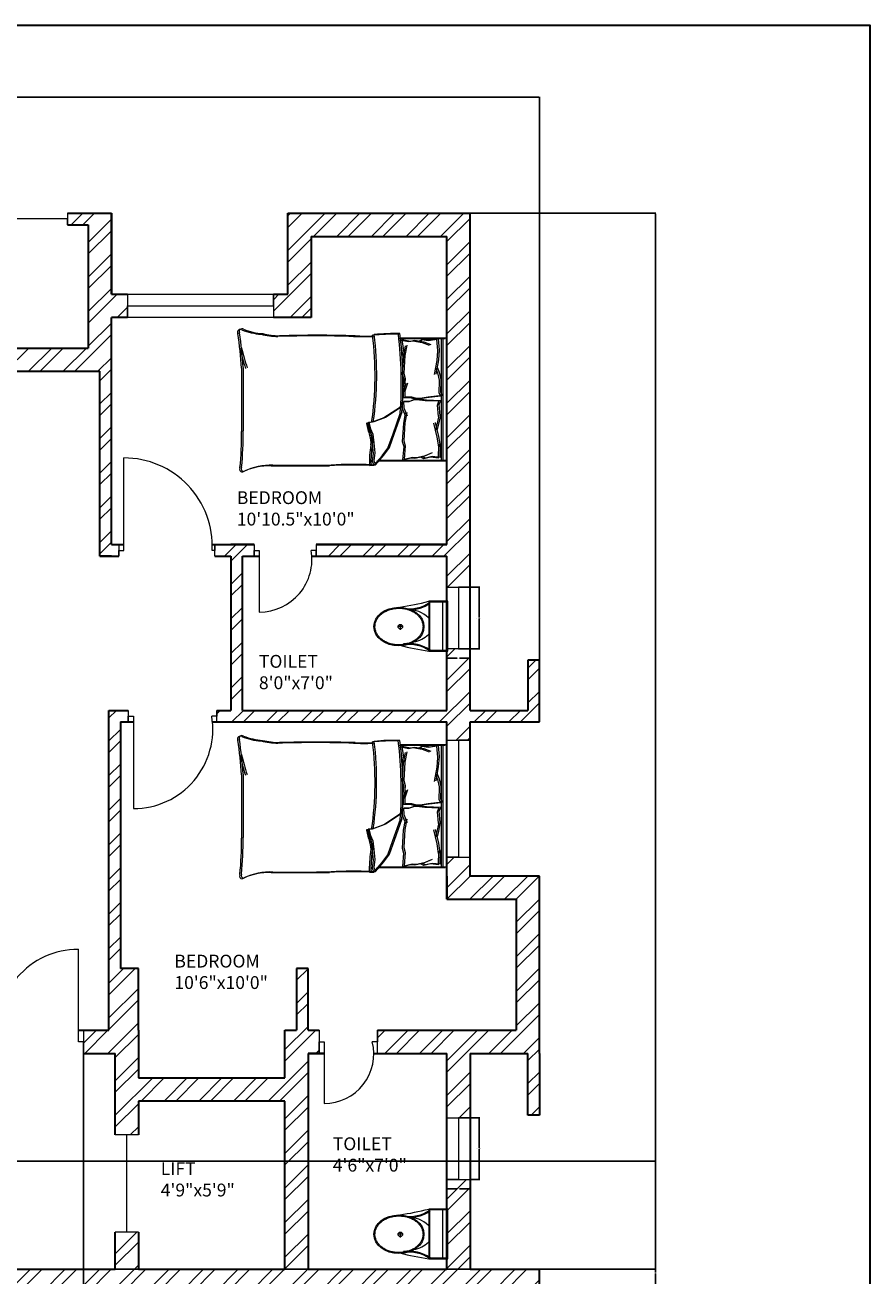
# Model space of a CAD drawing. Units: inches. Extents: x 1513 to 2170, y 1240 to 2288.
# Tile 10 of 10: x 1842 to 2170, y 1801 to 2288. Entities that reach past the tile are written whole.
import ezdxf

# ---------------------------------------------------------------- set-up
doc = ezdxf.new("R2010")
doc.units = ezdxf.units.IN
for name, color, linetype, lineweight in [('A-ANNO-DIMS', 2, 'Continuous', 18), ('A-ANNO-TTLB', 7, 'Continuous', 35), ('A-AREA-IDEN', 7, 'Continuous', 18), ('A-DOOR', 3, 'Continuous', 18), ('A-FLOR-FIXT', 9, 'Continuous', 18), ('A-FLOR-HRAL', 7, 'Continuous', 18), ('A-FURN', 8, 'Continuous', 18), ('A-GLAZ', 4, 'Continuous', 18), ('A-WALL', 7, 'Continuous', 35), ('A-WALL-PATT', 252, 'Continuous', 13)]:
    doc.layers.add(name, color=color, linetype=linetype, lineweight=lineweight)
doc.styles.get("Standard").update_dxf_attribs({"font": 'arial.ttf'})
doc.dimstyles.get("Standard").update_dxf_attribs({"dimtxt": 0.18, "dimasz": 0.18, "dimexe": 0.18, "dimexo": 0.0625, "dimgap": 0.09, "dimtad": 0, "dimtih": 1, "dimtoh": 1, "dimdec": 4, "dimzin": 0, "dimdsep": 46, "dimtxsty": 'Standard', "dimcen": 0.09, "dimadec": 0, "dimazin": 0, "dimtfac": 1, "dimtdec": 4, "dimtofl": 0, "dimtmove": 0, "dimatfit": 3, "dimfxl": 1, "dimtolj": 1, "dimtzin": 0, "dimarcsym": 0})

# ---------------------------------------------------------------- blocks, each defined once
blk = doc.blocks.new('A$C31115884')
for p, q in [((258, 466), (258, 523)), ((283, 498), (223, 498)), ((0, 200), (0, 0)), ((520, 200), (0, 200)), ((10, 190), (10, 10)), ((510, 190), (10, 190)), ((510, 10), (510, 190)), ((520, 0), (520, 200)), ((510, 54), (0, 54)), ((10, 10), (510, 10)), ((0, 0), (520, 0))]:
    blk.add_line(p, q)
blk.add_circle((256, 496), 23.6)
for centre, radius, start, end in [((2778, -205), 2807, 165.4549, 171.7133), ((-295, 403), 365, 324.2091, 9.3499), ((-295, 403), 375, 324.2091, 9.3499), ((139, 406), 293, 315.8436, 2.6563), ((806, 403), 375, 179.2036, 215.7909), ((806, 403), 365, 170.6501, 215.7909), ((3237, 905), 2807, 188.2867, 194.5451), ((384, 406), 293, 190.2774, 224.1564)]:
    blk.add_arc(centre, radius, start, end)
blk.add_ellipse((256, 510), major_axis=(0, -261), ratio=0.772727)
blk.add_open_spline([(256, 259), (263, 259), (270, 260), (288, 262), (299, 265), (320, 273), (330, 278), (350, 291), (360, 299), (378, 316), (386, 326), (402, 347), (409, 358), (421, 383), (427, 395), (436, 422), (440, 436), (445, 465), (447, 480), (448, 509), (448, 524), (445, 553), (443, 568), (436, 596), (432, 610), (422, 636), (416, 649), (402, 672), (395, 683), (379, 703), (370, 712), (351, 728), (341, 735), (321, 746), (310, 751), (289, 757), (278, 759), (256, 761), (245, 761), (223, 757), (212, 754), (191, 746), (181, 741), (161, 728), (151, 720), (133, 703), (125, 693), (110, 672), (103, 660), (90, 636), (85, 623), (76, 596), (72, 582), (67, 553), (66, 538), (64, 509), (65, 494), (68, 465), (70, 450), (77, 422), (81, 408), (91, 382), (97, 370), (111, 346), (118, 335), (135, 316), (144, 307), (162, 291), (172, 284), (193, 273), (203, 269), (225, 262), (236, 260), (250, 259), (253, 259), (256, 259)], degree=3, knots=[0, 0, 0, 0, 0.110105, 0.110105, 0.285049, 0.285049, 0.459994, 0.459994, 0.634938, 0.634938, 0.809882, 0.809882, 0.984827, 0.984827, 1.159771, 1.159771, 1.334715, 1.334715, 1.50966, 1.50966, 1.684604, 1.684604, 1.859549, 1.859549, 2.034493, 2.034493, 2.209437, 2.209437, 2.384382, 2.384382, 2.559326, 2.559326, 2.73427, 2.73427, 2.909215, 2.909215, 3.084159, 3.084159, 3.259103, 3.259103, 3.434048, 3.434048, 3.608992, 3.608992, 3.783936, 3.783936, 3.958881, 3.958881, 4.133825, 4.133825, 4.30877, 4.30877, 4.483714, 4.483714, 4.658658, 4.658658, 4.833603, 4.833603, 5.008547, 5.008547, 5.183491, 5.183491, 5.358436, 5.358436, 5.53338, 5.53338, 5.708324, 5.708324, 5.883269, 5.883269, 6.058213, 6.058213, 6.233158, 6.233158, 6.283185, 6.283185, 6.283185, 6.283185])
blk = doc.blocks.new('BED-DOUBLE')
for p, q in [((0, 51.27), (26.61, 51.27)), ((0, 51.27), (26.61, 51.27)), ((0.64, 51.49), (27.25, 51.49)), ((0.64, 51.49), (27.25, 51.49)), ((1.53, 3.48), (1.53, 51.27)), ((1.53, 3.48), (1.53, 51.27)), ((2.17, 3.7), (2.17, 51.49)), ((2.17, 3.7), (2.17, 51.49)), ((2.55, 50.11), (2.46, 44.71)), ((2.55, 50.11), (2.46, 44.71)), ((2.55, 50.11), (5.76, 49.73)), ((2.55, 50.11), (5.76, 49.73)), ((3.19, 50.34), (3.1, 44.94)), ((3.19, 50.34), (3.1, 44.94)), ((3.19, 50.34), (6.4, 49.96)), ((3.19, 50.34), (6.4, 49.96)), ((8.25, 49.31), (5.57, 48.13)), ((8.25, 49.31), (5.57, 48.13)), ((5.76, 49.73), (8.33, 50.33)), ((5.76, 49.73), (8.33, 50.33)), ((8.89, 49.54), (6.21, 48.36)), ((8.89, 49.54), (6.21, 48.36)), ((6.4, 49.96), (8.97, 50.56)), ((6.4, 49.96), (8.97, 50.56)), ((11.83, 50.11), (8.25, 49.31)), ((11.83, 50.11), (8.25, 49.31)), ((8.33, 50.33), (9.38, 49.82)), ((8.33, 50.33), (9.38, 49.82)), ((12.46, 50.34), (8.89, 49.54)), ((12.46, 50.34), (8.89, 49.54)), ((8.97, 50.56), (10.02, 50.04)), ((8.97, 50.56), (10.02, 50.04)), ((13.43, 49.92), (11.83, 50.11)), ((13.43, 49.92), (11.83, 50.11)), ((14.07, 50.15), (12.46, 50.34)), ((14.07, 50.15), (12.46, 50.34)), ((16.57, 50.7), (13.43, 49.92)), ((16.57, 50.7), (13.43, 49.92)), ((17.21, 50.93), (14.07, 50.15)), ((17.21, 50.93), (14.07, 50.15)), ((16.17, 45.57), (16.57, 50.7)), ((16.17, 45.57), (16.57, 50.7)), ((16.8, 45.8), (17.21, 50.93)), ((16.8, 45.8), (17.21, 50.93)), ((24.49, 49.16), (22.33, 46.22)), ((24.49, 49.16), (22.33, 46.22)), ((25.13, 49.39), (22.96, 46.45)), ((25.13, 49.39), (22.96, 46.45)), ((27.74, 52.87), (24.49, 49.16)), ((27.74, 52.87), (24.49, 49.16)), ((28.38, 53.1), (25.13, 49.39)), ((28.38, 53.1), (25.13, 49.39)), ((29.49, 52.95), (27.74, 52.87, 3.87)), ((29.49, 52.95), (27.74, 52.87, 3.87)), ((28.36, 51.33), (27.74, 52.87)), ((28.36, 51.33), (27.74, 52.87)), ((28.05, 48.23), (28.36, 51.33)), ((28.05, 48.23), (28.36, 51.33)), ((30.13, 53.18), (28.38, 53.1, 3.87)), ((30.13, 53.18), (28.38, 53.1, 3.87)), ((29, 51.56), (28.38, 53.1)), ((29, 51.56), (28.38, 53.1)), ((28.69, 48.46), (29, 51.56)), ((28.69, 48.46), (29, 51.56)), ((2.46, 44.71), (2.54, 45.71)), ((2.46, 44.71), (2.54, 45.71)), ((2.54, 45.71), (3.07, 41.92)), ((2.54, 45.71), (3.07, 41.92)), ((3.1, 44.94), (3.18, 45.94)), ((3.1, 44.94), (3.18, 45.94)), ((3.18, 45.94), (3.71, 42.14)), ((3.18, 45.94), (3.71, 42.14)), ((16.72, 43.61), (16.17, 45.57)), ((16.72, 43.61), (16.17, 45.57)), ((17.36, 43.84), (16.8, 45.8)), ((17.36, 43.84), (16.8, 45.8)), ((16.93, 36.83), (17.36, 43.84)), ((16.93, 36.83), (17.36, 43.84)), ((22.33, 46.22), (20.31, 40.65)), ((22.33, 46.22), (20.31, 40.65)), ((22.96, 46.45), (20.95, 40.87)), ((22.96, 46.45), (20.95, 40.87)), ((28.36, 44.36), (28.05, 48.23)), ((28.36, 44.36), (28.05, 48.23)), ((28.83, 40.96), (28.36, 44.36)), ((28.83, 40.95), (28.36, 44.36)), ((29, 44.59), (28.69, 48.46)), ((29, 44.59), (28.69, 48.46)), ((29.46, 41.18), (29, 44.59)), ((29.46, 41.18), (29, 44.59)), ((3.07, 41.92), (4.42, 36.5)), ((3.07, 41.92), (4.42, 36.5)), ((3.67, 39.2), (3.07, 37.14)), ((3.67, 39.2), (3.07, 37.14)), ((3.71, 42.14), (5.06, 36.72)), ((3.71, 42.14), (5.06, 36.72)), ((4.31, 39.43), (3.71, 37.36)), ((4.31, 39.43), (3.71, 37.36)), ((16.29, 36.6), (16.72, 43.61)), ((16.29, 36.6), (16.72, 43.61)), ((20.31, 40.65), (17.38, 32.31)), ((20.31, 40.65), (17.38, 32.31)), ((20.95, 40.87), (18.02, 32.54)), ((20.95, 40.87), (18.02, 32.54)), ((29.75, 38.94), (28.83, 40.96)), ((29.75, 38.94), (28.83, 40.95)), ((30.39, 39.17), (29.46, 41.18)), ((30.39, 39.17), (29.46, 41.18)), ((30.37, 36.46), (29.75, 38.94)), ((30.37, 36.46), (29.75, 38.94)), ((31.01, 36.69), (30.39, 39.17)), ((31.01, 36.69), (30.39, 39.17)), ((79.24, 15.06), (79.24, 39.68)), ((79.24, 15.06), (79.24, 39.68)), ((79.88, 15.29), (79.88, 39.91)), ((79.88, 15.29), (79.88, 39.91)), ((3.07, 37.14), (2.53, 34.21)), ((3.07, 37.14), (2.53, 34.21)), ((2.53, 34.21), (2.55, 33.88)), ((2.53, 34.21), (2.55, 33.88)), ((3.71, 37.36), (3.17, 34.43)), ((3.71, 37.36), (3.17, 34.43)), ((3.17, 34.43), (3.19, 34.11)), ((3.17, 34.43), (3.19, 34.11)), ((3.19, 34.11), (3.61, 29.69)), ((3.19, 34.11), (3.61, 29.68)), ((15.62, 32.57), (16.29, 36.6)), ((15.62, 32.57), (16.29, 36.6)), ((16.26, 32.79), (16.93, 36.83)), ((16.26, 32.79), (16.93, 36.83)), ((17.38, 30.26), (23.87, 34.45)), ((17.38, 30.26), (23.87, 34.45)), ((18.02, 30.49), (24.51, 34.68)), ((18.02, 30.49), (24.51, 34.68)), ((23.87, 34.45), (28.36, 36.15)), ((23.87, 34.45), (28.36, 36.15)), ((24.51, 34.68), (29, 36.38)), ((24.51, 34.68), (29, 36.38)), ((28.36, 36.15), (30.37, 36.46)), ((28.36, 36.15), (30.37, 36.46)), ((29, 36.38), (31.01, 36.69)), ((29, 36.38), (31.01, 36.69)), ((2.98, 29.46), (2.49, 27.98)), ((2.98, 29.46), (2.49, 27.98)), ((2.55, 33.88), (2.98, 29.46)), ((2.55, 33.88), (2.98, 29.46)), ((3.61, 29.69), (3.13, 28.21)), ((3.61, 29.68), (3.13, 28.21)), ((16.74, 30.75), (15.45, 33.82)), ((16.74, 30.75), (15.45, 33.82)), ((17.38, 30.98), (16.09, 34.05)), ((17.38, 30.98), (16.09, 34.05)), ((16.89, 28.3), (16.74, 30.75)), ((16.89, 28.3), (16.74, 30.75)), ((17.53, 28.53), (17.38, 30.98)), ((17.53, 28.53), (17.38, 30.98)), ((1.87, 25.98), (7.22, 26.56)), ((1.87, 25.98), (7.22, 26.56)), ((2.44, 24.54), (1.87, 25.98)), ((2.44, 24.54), (1.87, 25.98)), ((2.3, 20.09), (2.44, 24.54)), ((2.3, 20.09), (2.44, 24.54)), ((2.49, 27.98), (7.86, 27.73)), ((2.49, 27.98), (7.86, 27.73)), ((2.51, 26.21), (7.86, 26.79)), ((2.51, 26.21), (7.86, 26.79)), ((3.08, 24.77), (2.51, 26.21)), ((3.08, 24.77), (2.51, 26.21)), ((2.94, 20.32), (3.08, 24.77)), ((2.94, 20.32), (3.08, 24.77)), ((3.13, 28.21), (8.5, 27.96)), ((3.13, 28.21), (8.5, 27.96)), ((7.22, 26.56), (10.4, 27.14)), ((7.22, 26.56), (10.4, 27.14)), ((7.86, 27.73), (11.07, 27.36)), ((7.86, 27.73), (11.07, 27.36)), ((7.86, 26.79), (11.04, 27.37)), ((7.86, 26.79), (11.04, 27.37)), ((8.5, 27.96), (11.71, 27.58)), ((8.5, 27.96), (11.71, 27.58)), ((10.4, 27.14), (11.7, 27.14)), ((10.4, 27.14), (11.7, 27.14)), ((11.04, 27.37), (12.34, 27.37)), ((11.04, 27.37), (12.34, 27.37)), ((11.07, 27.36), (12.37, 27.44)), ((11.07, 27.36), (12.37, 27.44)), ((11.7, 27.14), (13.58, 26.56)), ((11.7, 27.14), (13.58, 26.56)), ((11.71, 27.58), (13.01, 27.67)), ((11.71, 27.58), (13.01, 27.67)), ((12.34, 27.37), (14.22, 26.79)), ((12.34, 27.37), (14.22, 26.79)), ((12.37, 27.44), (14.21, 28.13)), ((12.37, 27.44), (14.21, 28.13)), ((13.01, 27.67), (14.85, 28.36)), ((13.01, 27.67), (14.85, 28.36)), ((13.58, 26.56), (16.26, 26.56)), ((13.58, 26.56), (16.26, 26.56)), ((14.21, 28.13), (16.89, 28.3)), ((14.21, 28.13), (16.89, 28.3)), ((14.22, 26.79), (16.9, 26.79)), ((14.22, 26.79), (16.9, 26.79)), ((14.85, 28.36), (17.53, 28.53)), ((14.85, 28.36), (17.53, 28.53)), ((16.9, 24.33), (15.81, 21.19)), ((16.9, 24.33), (15.81, 21.19)), ((16.17, 19.39), (16.57, 24.52)), ((16.17, 19.38), (16.57, 24.52)), ((16.26, 26.56), (16.26, 24.1)), ((16.26, 26.56), (16.26, 24.1)), ((16.8, 19.61), (17.21, 24.75)), ((16.8, 19.61), (17.21, 24.74)), ((16.9, 26.79), (16.9, 24.33)), ((16.9, 26.79), (16.9, 24.33)), ((2.3, 19.77), (2.3, 20.09)), ((2.3, 19.77), (2.3, 20.09)), ((3.02, 16.88), (2.3, 19.77)), ((3.02, 16.88), (2.3, 19.77)), ((2.94, 20), (2.94, 20.32)), ((2.94, 20), (2.94, 20.32)), ((3.66, 17.11), (2.94, 20)), ((3.66, 17.11), (2.94, 20)), ((16.26, 24.1), (15.17, 20.96)), ((16.26, 24.1), (15.17, 20.96)), ((17.36, 17.65), (16.8, 19.61)), ((17.36, 17.65), (16.8, 19.61)), ((3.75, 14.86), (3.02, 16.88)), ((3.75, 14.86), (3.02, 16.88)), ((3.31, 12.11), (4.32, 17.6)), ((3.31, 12.11), (4.32, 17.6)), ((4.39, 15.08), (3.66, 17.11)), ((4.39, 15.08), (3.66, 17.11)), ((3.95, 12.34), (4.96, 17.83)), ((3.95, 12.34), (4.96, 17.83)), ((16.72, 17.42), (16.17, 19.39)), ((16.72, 17.42), (16.17, 19.38)), ((16.29, 10.41), (16.72, 17.42)), ((16.29, 10.41), (16.72, 17.42)), ((16.93, 10.64), (17.36, 17.65)), ((16.93, 10.64), (17.36, 17.65)), ((3.02, 8.29), (3.31, 12.11)), ((3.02, 8.29), (3.31, 12.11)), ((3.66, 8.51), (3.95, 12.34)), ((3.66, 8.51), (3.95, 12.34)), ((15.62, 6.38), (16.29, 10.41)), ((15.62, 6.38), (16.29, 10.41)), ((16.26, 6.61), (16.93, 10.64)), ((16.26, 6.61), (16.93, 10.64)), ((16.29, 10.41), (16.61, 9.28)), ((16.29, 10.41), (16.61, 9.28)), ((16.93, 10.64), (17.25, 9.51)), ((16.93, 10.64), (17.25, 9.51)), ((3.01, 8.18), (3.02, 8.29)), ((3.01, 8.18), (3.02, 8.29)), ((3.33, 3.9), (3.01, 8.18)), ((3.33, 3.9), (3.01, 8.18)), ((3.64, 8.41), (3.66, 8.51)), ((3.64, 8.41), (3.66, 8.51)), ((3.97, 4.13), (3.64, 8.41)), ((3.97, 4.13), (3.64, 8.41)), ((8.95, 5.05), (6.2, 6.06)), ((8.95, 5.05), (6.2, 6.06)), ((9.59, 5.28), (6.84, 6.29)), ((9.59, 5.28), (6.84, 6.29)), ((12.57, 4.47), (8.95, 5.05)), ((12.57, 4.47), (8.95, 5.05)), ((13.21, 4.7), (9.59, 5.28)), ((13.21, 4.7), (9.59, 5.28)), ((14.8, 4.99), (13.21, 4.7)), ((14.8, 4.99), (13.21, 4.7)), ((17.98, 4.41), (14.8, 4.99)), ((17.98, 4.41), (14.8, 4.99)), ((16.61, 9.28), (17.34, 4.18)), ((16.61, 9.28), (17.34, 4.18)), ((17.25, 9.51), (17.98, 4.41)), ((17.25, 9.51), (17.98, 4.41)), ((18.11, 3.48), (0, 3.48)), ((18.11, 3.48), (0, 3.48)), ((18.75, 3.7), (0.64, 3.7)), ((18.75, 3.7), (0.64, 3.7)), ((3.31, 3.9), (6.49, 4.47)), ((3.31, 3.9), (6.49, 4.47)), ((3.95, 4.12), (7.13, 4.7)), ((3.95, 4.12), (7.13, 4.7)), ((6.49, 4.47), (9.1, 4.04)), ((6.49, 4.47), (9.1, 4.04)), ((7.13, 4.7), (9.74, 4.27)), ((7.13, 4.7), (9.74, 4.27)), ((9.1, 4.04), (10.11, 4.62)), ((9.1, 4.04), (10.11, 4.62)), ((9.74, 4.27), (10.75, 4.85)), ((9.74, 4.27), (10.75, 4.85)), ((14.16, 4.76), (12.57, 4.47)), ((14.16, 4.76), (12.57, 4.47)), ((17.34, 4.18), (14.16, 4.76)), ((17.34, 4.18), (14.16, 4.76))]:
    blk.add_line(p, q)
for centre, radius, start, end in [((68.66, 76.16), 23.07, 267.4714, 296.4681), ((68.66, 76.16), 23.07, 267.4714, 296.4681), ((69.3, 76.39), 23.07, 267.4714, 296.4681), ((69.3, 76.39), 23.07, 267.4714, 296.4681), ((78.87, 54.41), 1.1, 332.6588, 86.02), ((78.87, 54.41), 1.1, 332.6588, 86.02), ((212.27, 41.15), 133.04, 174.4998, 180.6351), ((212.27, 41.15), 133.04, 174.4998, 180.6351), ((79.51, 54.64), 1.1, 332.6588, 86.02), ((79.51, 54.64), 1.1, 332.6588, 86.02), ((212.91, 41.38), 133.04, 174.4998, 180.6351), ((212.91, 41.38), 133.04, 174.4998, 180.6351), ((-6.66, 51.33), 36.18, 349.8763, 2.5657), ((-6.66, 51.33), 36.18, 349.8763, 2.5657), ((36.31, 182.27), 129.5, 266.9791, 273.8365), ((36.31, 182.27), 129.5, 266.9791, 273.8365), ((-6.02, 51.56), 36.18, 349.8763, 2.5657), ((-6.02, 51.56), 36.18, 349.8763, 2.5657), ((36.95, 182.5), 129.5, 266.9791, 273.8365), ((36.95, 182.5), 129.5, 266.9791, 273.8365), ((67.82, -4508.74), 4561.86, 90.00217, 90.28689), ((67.82, -4508.74), 4561.86, 90.00217, 90.28689), ((68.46, -4508.51), 4561.86, 90.00217, 90.28689), ((68.46, -4508.51), 4561.86, 90.00217, 90.28689), ((35.06, 43.74), 6.22, 168.6608, 203.7384), ((35.06, 43.74), 6.22, 168.6608, 203.7384), ((35.7, 43.97), 6.22, 168.6608, 203.7384), ((35.7, 43.97), 6.22, 168.6608, 203.7384), ((1.48, 31.15), 29.65, 10.6617, 19.8806), ((1.48, 31.15), 29.65, 10.6617, 19.8806), ((2.12, 31.38), 29.65, 10.6617, 19.8806), ((2.12, 31.38), 29.65, 10.6617, 19.8806), ((156.31, 17.76), 129.02, 171.7845, 186.9006), ((156.31, 17.76), 129.02, 171.7845, 186.9006), ((156.95, 17.99), 129.02, 171.7845, 186.9006), ((156.95, 17.98), 129.02, 171.7845, 186.9006), ((30.44, 36.64), 0.185, 250.2464, 1.1377), ((30.44, 36.64), 0.185, 250.2464, 1.1377), ((31.08, 36.87), 0.185, 250.2464, 1.1377), ((31.08, 36.87), 0.185, 250.2464, 1.1377), ((182.05, 21.36), 164.97, 176.0865, 186.7821), ((182.05, 21.36), 164.97, 176.0865, 186.7821), ((182.69, 21.59), 164.97, 176.0865, 186.7821), ((182.69, 21.59), 164.97, 176.0865, 186.7821), ((-23.72, -17.22), 106.46, 13.3832, 17.7053), ((-23.72, -17.22), 106.46, 13.3832, 17.7053), ((-23.08, -16.99), 106.46, 13.3832, 17.7053), ((-23.08, -16.99), 106.46, 13.3832, 17.7053), ((200.83, 21.43), 121.76, 182.9958, 189.4091), ((200.83, 21.43), 121.76, 182.9958, 189.4091), ((201.47, 21.66), 121.76, 182.9958, 189.4091), ((201.47, 21.66), 121.76, 182.9958, 189.4091), ((20.09, 85.16), 83.31, 268.7218, 275.604), ((20.09, 85.16), 83.31, 268.7218, 275.604), ((20.73, 85.39), 83.31, 268.7218, 275.604), ((20.73, 85.39), 83.31, 268.7218, 275.604), ((31.17, -167.31), 170.11, 88.4762, 91.0082), ((31.17, -167.31), 170.11, 88.4762, 91.0082), ((31.81, -167.08), 170.11, 88.4762, 91.0082), ((31.81, -167.08), 170.11, 88.4762, 91.0082), ((50.61, 484.82), 482.31, 268.2277, 271.7185), ((50.61, 484.82), 482.31, 268.2277, 271.7185), ((51.25, 485.05), 482.31, 268.2277, 271.7185), ((51.25, 485.05), 482.31, 268.2277, 271.7185), ((64.51, -26.9), 29.63, 76.0648, 88.9113), ((64.51, -26.9), 29.63, 76.0648, 88.9113), ((65.15, -26.67), 29.63, 76.0648, 88.9113), ((65.15, -26.67), 29.63, 76.0648, 88.9113), ((70.27, -21.66), 23.56, 67.9751, 86.652), ((70.27, -21.66), 23.56, 67.9751, 86.652), ((70.91, -21.43), 23.56, 67.9751, 86.652), ((70.91, -21.43), 23.56, 67.9751, 86.652), ((79.71, 1.09), 1.09, 236.1736, 23.4781), ((79.71, 1.09), 1.09, 236.1736, 23.4781), ((80.35, 1.32), 1.09, 236.1736, 23.4781), ((80.35, 1.32), 1.09, 236.1736, 23.4781)]:
    blk.add_arc(centre, radius, start, end)
blk = doc.blocks.new('WIN-24')
for p, q in [((0, 24), (9, 24)), ((9, 24), (4.5, 24)), ((4.5, 24), (4.5, 0)), ((4.5, 0), (0, 0)), ((0, 0), (9, 0))]:
    blk.add_line(p, q)
blk = doc.blocks.new('WIN-24-ALT')
for p, q in [((4.5, 24), (0, 24)), ((0, 24), (9, 24)), ((4.5, 0), (4.5, 24)), ((9, 0), (0, 0)), ((0, 0), (4.5, 0))]:
    blk.add_line(p, q)
blk = doc.blocks.new('*D13')
at = {"layer": 'A-ANNO-DIMS', "color": 0, "lineweight": -2, "transparency": 16777216}
for p, q in [((2014.91, 1862.4), (2018.63, 1862.4)), ((2018.45, 1862.22), (2018.45, 1850.58)), ((2018.45, 1838.58), (2018.45, 1850.22)), ((2014.91, 1838.4), (2018.63, 1838.4))]:
    blk.add_line(p, q, dxfattribs=at)
at = {"layer": 'A-ANNO-DIMS', "color": 0, "transparency": 16777216}
for points in [[(2018.42, 1862.22), (2018.48, 1862.22), (2018.45, 1862.4)], [(2018.42, 1838.58), (2018.48, 1838.58), (2018.45, 1838.4)]]:
    blk.add_solid(points, dxfattribs=at)
at = {"layer": 'Defpoints', "color": 0, "transparency": 16777216}
for p in [(2014.85, 1862.4), (2018.45, 1862.4), (2014.85, 1838.4)]:
    blk.add_point(p, dxfattribs=at)
at = {"layer": 'A-ANNO-DIMS', "color": 0, "transparency": 16777216, "insert": (2018.45, 1850.4), "char_height": 0.18, "attachment_point": 5}
blk.add_mtext('\\A1;WINDOW 24 TYP.', dxfattribs=at)
blk = doc.blocks.new('*D14')
at = {"layer": 'A-ANNO-DIMS', "color": 0, "lineweight": -2, "transparency": 16777216}
for p, q in [((2005.85, 1838.34), (2005.85, 1834.62)), ((2006.03, 1834.8), (2009.89, 1834.8)), ((2014.67, 1834.8), (2010.81, 1834.8)), ((2014.85, 1838.34), (2014.85, 1834.62))]:
    blk.add_line(p, q, dxfattribs=at)
at = {"layer": 'A-ANNO-DIMS', "color": 0, "transparency": 16777216}
for points in [[(2006.03, 1834.83), (2006.03, 1834.77), (2005.85, 1834.8)], [(2014.67, 1834.83), (2014.67, 1834.77), (2014.85, 1834.8)]]:
    blk.add_solid(points, dxfattribs=at)
at = {"layer": 'Defpoints', "color": 0, "transparency": 16777216}
for p in [(2005.85, 1838.4), (2014.85, 1838.4), (2014.85, 1834.8)]:
    blk.add_point(p, dxfattribs=at)
at = {"layer": 'A-ANNO-DIMS', "color": 0, "transparency": 16777216, "insert": (2010.35, 1834.8), "char_height": 0.18, "attachment_point": 5}
blk.add_mtext('\\A1;9 TYP.', dxfattribs=at)
blk = doc.blocks.new('*D15')
at = {"layer": 'A-ANNO-DIMS', "color": 0, "lineweight": -2, "transparency": 16777216}
for p, q in [((2014.91, 2068.9), (2018.63, 2068.9)), ((2018.45, 2068.72), (2018.45, 2057.09)), ((2018.45, 2045.08), (2018.45, 2056.72)), ((2014.91, 2044.9), (2018.63, 2044.9))]:
    blk.add_line(p, q, dxfattribs=at)
at = {"layer": 'A-ANNO-DIMS', "color": 0, "transparency": 16777216}
for points in [[(2018.42, 2068.72), (2018.48, 2068.72), (2018.45, 2068.9)], [(2018.42, 2045.08), (2018.48, 2045.08), (2018.45, 2044.9)]]:
    blk.add_solid(points, dxfattribs=at)
at = {"layer": 'Defpoints', "color": 0, "transparency": 16777216}
for p in [(2014.85, 2068.9), (2014.85, 2044.9), (2018.45, 2044.9)]:
    blk.add_point(p, dxfattribs=at)
at = {"layer": 'A-ANNO-DIMS', "color": 0, "transparency": 16777216, "insert": (2018.45, 2056.9), "char_height": 0.18, "attachment_point": 5}
blk.add_mtext('\\A1;ALT WINDOW 24 TYP.', dxfattribs=at)
blk = doc.blocks.new('*D16')
at = {"layer": 'A-ANNO-DIMS', "color": 0, "lineweight": -2, "transparency": 16777216}
for p, q in [((2005.85, 2044.84), (2005.85, 2041.12)), ((2014.85, 2044.84), (2014.85, 2041.12)), ((2006.03, 2041.3), (2009.89, 2041.3)), ((2014.67, 2041.3), (2010.81, 2041.3))]:
    blk.add_line(p, q, dxfattribs=at)
at = {"layer": 'A-ANNO-DIMS', "color": 0, "transparency": 16777216}
for points in [[(2006.03, 2041.33), (2006.03, 2041.27), (2005.85, 2041.3)], [(2014.67, 2041.33), (2014.67, 2041.27), (2014.85, 2041.3)]]:
    blk.add_solid(points, dxfattribs=at)
at = {"layer": 'Defpoints', "color": 0, "transparency": 16777216}
for p in [(2005.85, 2044.9), (2014.85, 2044.9), (2005.85, 2041.3)]:
    blk.add_point(p, dxfattribs=at)
at = {"layer": 'A-ANNO-DIMS', "color": 0, "transparency": 16777216, "insert": (2010.35, 2041.3), "char_height": 0.18, "attachment_point": 5}
blk.add_mtext('\\A1;9 TYP.', dxfattribs=at)
blk = doc.blocks.new('*D25')
at = {"layer": 'A-ANNO-DIMS', "color": 0, "lineweight": -2, "transparency": 16777216}
for p, q in [((1578.87, 2040.54), (1578.87, 2259.81)), ((1579.05, 2259.63), (1810.07, 2259.63)), ((2041.67, 2259.63), (1810.65, 2259.63)), ((2041.85, 2040.54), (2041.85, 2259.81))]:
    blk.add_line(p, q, dxfattribs=at)
at = {"layer": 'A-ANNO-DIMS', "color": 0, "transparency": 16777216}
for points in [[(1579.05, 2259.66), (1579.05, 2259.6), (1578.87, 2259.63)], [(2041.67, 2259.66), (2041.67, 2259.6), (2041.85, 2259.63)]]:
    blk.add_solid(points, dxfattribs=at)
at = {"layer": 'Defpoints', "color": 0, "transparency": 16777216}
for p in [(2041.85, 2259.63), (1578.87, 2040.48), (2041.85, 2040.48)]:
    blk.add_point(p, dxfattribs=at)
at = {"layer": 'A-ANNO-DIMS', "color": 0, "transparency": 16777216, "insert": (1810.36, 2259.63), "char_height": 0.18, "attachment_point": 5}
blk.add_mtext('\\A1;463', dxfattribs=at)
blk = doc.blocks.new('*D26')
at = {"layer": 'A-ANNO-DIMS', "color": 0, "lineweight": -2, "transparency": 16777216}
for p, q in [((2014.91, 2214.48), (2087.18, 2214.48)), ((2087, 2214.3), (2087, 1802.16)), ((2087, 1389.66), (2087, 1801.8)), ((1937.43, 1389.48), (2087.18, 1389.48))]:
    blk.add_line(p, q, dxfattribs=at)
at = {"layer": 'A-ANNO-DIMS', "color": 0, "transparency": 16777216}
for points in [[(2086.97, 2214.3), (2087.03, 2214.3), (2087, 2214.48)], [(2086.97, 1389.66), (2087.03, 1389.66), (2087, 1389.48)]]:
    blk.add_solid(points, dxfattribs=at)
at = {"layer": 'Defpoints', "color": 0, "transparency": 16777216}
for p in [(2014.85, 2214.48), (2087, 2214.48), (1937.37, 1389.48)]:
    blk.add_point(p, dxfattribs=at)
at = {"layer": 'A-ANNO-DIMS', "color": 0, "transparency": 16777216, "insert": (2087, 1801.98), "char_height": 0.18, "attachment_point": 5}
blk.add_mtext('\\A1;825', dxfattribs=at)
blk = doc.blocks.new('*D35')
at = {"layer": 'A-ANNO-DIMS', "color": 0, "lineweight": -2, "transparency": 16777216}
for p, q in [((1754.53, 1845.48), (2087.18, 1845.48)), ((2087, 1845.3), (2087, 1824.66)), ((2087, 1803.66), (2087, 1824.3)), ((1754.53, 1803.48), (2087.18, 1803.48))]:
    blk.add_line(p, q, dxfattribs=at)
at = {"layer": 'A-ANNO-DIMS', "color": 0, "transparency": 16777216}
for points in [[(2086.97, 1845.3), (2087.03, 1845.3), (2087, 1845.48)], [(2086.97, 1803.66), (2087.03, 1803.66), (2087, 1803.48)]]:
    blk.add_solid(points, dxfattribs=at)
at = {"layer": 'Defpoints', "color": 0, "transparency": 16777216}
for p in [(1754.46, 1845.48), (2087, 1845.48), (1754.46, 1803.48)]:
    blk.add_point(p, dxfattribs=at)
at = {"layer": 'A-ANNO-DIMS', "color": 0, "transparency": 16777216, "insert": (2087, 1824.48), "char_height": 0.18, "attachment_point": 5}
blk.add_mtext('\\A1;42', dxfattribs=at)
blk = doc.blocks.new('*D36')
at = {"layer": 'A-ANNO-DIMS', "color": 0, "lineweight": -2, "transparency": 16777216}
for p, q in [((1829.49, 1887.42), (1829.49, 1344.15)), ((1864.51, 1887.42), (1864.51, 1344.15)), ((1829.67, 1344.33), (1846.61, 1344.33)), ((1864.33, 1344.33), (1847.39, 1344.33))]:
    blk.add_line(p, q, dxfattribs=at)
at = {"layer": 'A-ANNO-DIMS', "color": 0, "transparency": 16777216}
for points in [[(1829.67, 1344.36), (1829.67, 1344.3), (1829.49, 1344.33)], [(1864.33, 1344.36), (1864.33, 1344.3), (1864.51, 1344.33)]]:
    blk.add_solid(points, dxfattribs=at)
at = {"layer": 'Defpoints', "color": 0, "transparency": 16777216}
for p in [(1829.49, 1887.48), (1864.51, 1887.48), (1864.51, 1344.33)]:
    blk.add_point(p, dxfattribs=at)
at = {"layer": 'A-ANNO-DIMS', "color": 0, "transparency": 16777216, "insert": (1847, 1344.33), "char_height": 0.18, "attachment_point": 5}
blk.add_mtext('\\A1;35.02', dxfattribs=at)

msp = doc.modelspace()

# ---------------------------------------------------------------- hatches: boundary and pattern name
at = {"layer": 'A-WALL-PATT'}
h = msp.add_hatch(dxfattribs=at)
h.set_pattern_fill('ANSI32', color=256)
h.paths.add_polyline_path([(1744.852, 2209.98), (1762.042, 2209.98), (1762.042, 2214.48), (1715.345, 2214.48), (1715.345, 2205.48), (1735.852, 2205.48), (1735.852, 2161.98), (1733.253, 2161.98), (1719.866, 2161.98), (1719.866, 2112.429), (1724.366, 2112.429), (1724.366, 2152.98), (1762.042, 2152.98), (1870.852, 2152.98), (1870.852, 2080.98), (1875.352, 2080.98), (1878.245, 2080.98), (1878.245, 2083.23), (1878.245, 2085.48), (1875.352, 2085.48), (1875.352, 2173.929), (1881.628, 2173.929), (1881.628, 2178.429), (1881.628, 2182.929), (1875.352, 2182.929), (1875.352, 2214.48), (1858.335, 2214.48), (1858.335, 2209.98), (1866.352, 2209.98), (1866.352, 2161.98), (1762.042, 2161.98), (1744.852, 2161.98)])
h.paths.add_polyline_path([(2014.852, 2214.48), (1944.011, 2214.48), (1944.011, 2182.929), (1938.347, 2182.929), (1938.347, 2173.929), (1953.011, 2173.929), (1953.011, 2182.929), (1953.011, 2205.48), (2005.852, 2205.48), (2005.852, 2085.48), (1955.061, 2085.48), (1955.061, 2080.98), (2005.852, 2080.98), (2005.852, 2068.903), (2014.852, 2068.903)])
h.paths.add_polyline_path([(2014.852, 2044.903), (2005.852, 2044.903), (2005.852, 2020.98), (1926.352, 2020.98), (1926.352, 2080.98), (1930.882, 2080.98), (1930.882, 2083.23), (1930.882, 2085.48), (1921.852, 2085.48), (1915.536, 2085.48), (1915.536, 2083.23), (1915.536, 2080.98), (1921.852, 2080.98), (1921.852, 2020.98), (1916.378, 2020.98), (1916.378, 2018.73), (1916.378, 2016.48), (2005.852, 2016.48), (2005.852, 2009.442), (2014.852, 2009.442), (2014.852, 2016.48), (2029.852, 2016.48), (2041.852, 2016.48), (2041.852, 2040.48), (2037.352, 2040.48), (2037.352, 2036.595), (2037.352, 2020.98), (2014.852, 2020.98)])
h.paths.add_polyline_path([(2041.852, 1956.48), (2014.852, 1956.48), (2014.852, 1963.797), (2005.852, 1963.797), (2005.852, 1947.48), (2032.852, 1947.48), (2032.852, 1896.48), (1978.852, 1896.48), (1978.852, 1891.98), (1978.852, 1887.48), (2005.852, 1887.48), (2005.852, 1862.401), (2014.852, 1862.401), (2014.852, 1887.48), (2037.352, 1887.48), (2037.352, 1863.48), (2041.852, 1863.48), (2041.852, 1887.48), (2041.852, 1896.48)], flags=17)
h.paths.add_polyline_path([(1885.852, 1896.48), (1885.852, 1920.48), (1878.866, 1920.48), (1878.866, 2016.48), (1881.925, 2016.48), (1881.925, 2018.73), (1881.925, 2020.98), (1874.366, 2020.98), (1874.366, 1896.48), (1864.508, 1896.48), (1864.508, 1887.48), (1876.852, 1887.48), (1876.852, 1855.773), (1885.852, 1855.773), (1885.852, 1868.947), (1942.852, 1868.947), (1942.852, 1803.48), (1885.852, 1803.48), (1885.852, 1817.861), (1876.852, 1817.861), (1876.852, 1803.48), (1825.976, 1803.48), (1825.976, 1798.98), (1825.976, 1794.48), (1832.366, 1794.48), (1832.366, 1663.98), (1832.366, 1659.48), (1841.939, 1659.48), (1841.939, 1661.73), (1841.939, 1663.98), (1836.866, 1663.98), (1836.866, 1794.48), (1992.866, 1794.48), (2005.852, 1794.48), (2005.852, 1784.304), (2010.352, 1784.304), (2014.852, 1784.304), (2014.852, 1794.48), (2041.852, 1794.48), (2041.852, 1803.48), (2014.852, 1803.48), (2014.852, 1838.401), (2005.852, 1838.401), (2005.852, 1803.48), (1951.852, 1803.48), (1951.852, 1887.48), (1956.114, 1887.48), (1956.114, 1891.98), (1956.114, 1896.48), (1951.852, 1896.48), (1951.852, 1920.48), (1947.352, 1920.48), (1947.352, 1896.48), (1942.852, 1896.48), (1942.852, 1877.947), (1885.852, 1877.947)])

# ---------------------------------------------------------------- linework, layer by layer
at = {"layer": 'A-ANNO-TTLB'}
msp.add_lwpolyline([(1513.071, 2287.731), (2170.435, 2287.731), (2170.435, 1239.669), (1513.071, 1239.669)], close=True, dxfattribs=at)
at = {"layer": 'A-DOOR'}
for p, q in [((1880.245, 2083.23), (1880.245, 2119.23)), ((1878.245, 2085.48), (1878.245, 2080.98)), ((1878.245, 2080.98), (1878.245, 2083.23)), ((1878.245, 2083.23), (1880.245, 2083.23)), ((1915.536, 2083.23), (1914.536, 2083.23)), ((1915.536, 2080.98), (1915.536, 2085.48)), ((1915.536, 2085.48), (1915.536, 2083.23)), ((1930.882, 2085.48), (1930.882, 2080.98)), ((1930.882, 2080.98), (1930.882, 2083.23)), ((1930.882, 2083.23), (1932.882, 2083.23)), ((1932.882, 2083.23), (1932.882, 2059.23)), ((1955.061, 2083.23), (1953.061, 2083.23)), ((1955.061, 2085.48), (1955.061, 2080.98)), ((1955.061, 2080.98), (1955.061, 2083.23)), ((1881.925, 2020.98), (1881.925, 2016.48)), ((1916.378, 2016.48), (1916.378, 2020.98)), ((1916.378, 2020.98), (1916.378, 2018.73)), ((1881.925, 2016.48), (1881.925, 2018.73)), ((1881.925, 2018.73), (1883.925, 2018.73)), ((1883.925, 2018.73), (1883.925, 1982.73)), ((1916.378, 2018.73), (1914.378, 2018.73)), ((1862.508, 1891.98), (1862.508, 1927.98)), ((1864.508, 1896.48), (1864.508, 1887.48)), ((1956.114, 1896.48), (1956.114, 1887.48)), ((1978.852, 1887.48), (1978.852, 1896.48)), ((1978.852, 1896.48), (1978.852, 1891.98)), ((1864.508, 1891.98), (1862.508, 1891.98)), ((1864.508, 1887.48), (1864.508, 1891.98)), ((1956.114, 1887.48), (1956.114, 1891.98)), ((1956.114, 1891.98), (1958.114, 1891.98)), ((1958.114, 1891.98), (1958.114, 1867.98)), ((1978.852, 1891.98), (1976.852, 1891.98)), ((1977.428, 1887.48), (1978.852, 1887.48)), ((1885.852, 1855.773), (1876.852, 1855.773)), ((1881.352, 1817.861), (1881.352, 1855.773)), ((1885.852, 1817.861), (1876.852, 1817.861))]:
    msp.add_line(p, q, dxfattribs=at)
for centre, radius, start, end in [((1880.245, 2084.898), 34.332, 357.21457, 90), ((1932.882, 2079.712), 20.483, 270, 9.88807), ((1883.925, 2013.61), 30.881, 270, 9.54205), ((1862.508, 1896.616), 31.363, 90, 188.50132), ((1958.114, 1887.294), 19.315, 270, 14.03893)]:
    msp.add_arc(centre, radius, start, end, dxfattribs=at)
at = {"layer": 'A-FLOR-HRAL'}
for p, q in [((1858.335, 2214.48), (1858.335, 2209.98)), ((1858.335, 2212.23), (1768.065, 2212.23)), ((1858.335, 2209.98), (1858.335, 2212.23))]:
    msp.add_line(p, q, dxfattribs=at)
at = {"layer": 'A-FURN'}
for p, q in [((2005.852, 2118.21), (2005.852, 2166)), ((2005.852, 2117.981), (2005.213, 2117.981))]:
    msp.add_line(p, q, dxfattribs=at)
at = {"layer": 'A-GLAZ'}
for p, q in [((1881.628, 2182.929), (1881.628, 2173.929)), ((1881.628, 2182.929), (1938.347, 2182.929)), ((1938.347, 2178.429), (1938.347, 2182.929)), ((1938.347, 2182.929), (1938.347, 2173.929)), ((1881.628, 2173.929), (1881.628, 2178.429)), ((1881.628, 2178.429), (1938.347, 2178.429)), ((1938.347, 2173.929), (1881.628, 2173.929)), ((2005.852, 2009.442), (2014.852, 2009.442)), ((2014.852, 2009.442), (2010.352, 2009.442)), ((2010.352, 2009.442), (2010.352, 1963.797)), ((2010.352, 1963.797), (2005.852, 1963.797)), ((2005.852, 1963.797), (2014.852, 1963.797))]:
    msp.add_line(p, q, dxfattribs=at)
at = {"layer": 'A-WALL'}
for p, q in [((1858.335, 2214.48), (1875.352, 2214.48)), ((1875.352, 2214.48), (1875.352, 2182.929)), ((1875.352, 2182.929), (1875.352, 2214.48)), ((1944.011, 2182.929), (1944.011, 2214.48)), ((1944.011, 2214.48), (2014.852, 2214.48)), ((2014.852, 2020.98), (2014.852, 2214.48)), ((1858.335, 2209.98), (1866.352, 2209.98)), ((1866.352, 2209.98), (1866.352, 2161.98)), ((1953.011, 2205.48), (2005.852, 2205.48)), ((1953.011, 2205.48), (1953.011, 2182.929)), ((2005.852, 2085.48), (2005.852, 2205.48)), ((1875.352, 2182.929), (1881.628, 2182.929)), ((1938.347, 2182.929), (1944.011, 2182.929)), ((1953.011, 2182.929), (1953.011, 2173.929)), ((1875.352, 2085.48), (1875.352, 2173.929)), ((1881.628, 2173.929), (1875.352, 2173.929)), ((1953.011, 2173.929), (1938.347, 2173.929)), ((1762.042, 2161.98), (1866.352, 2161.98)), ((1875.352, 2152.98), (1875.352, 2161.98)), ((1762.042, 2152.98), (1870.852, 2152.98)), ((1870.852, 2080.98), (1870.852, 2152.98)), ((1875.352, 2085.48), (1880.245, 2085.48)), ((1914.572, 2085.48), (1930.882, 2085.48)), ((1930.882, 2085.48), (1921.852, 2085.48)), ((2005.852, 2085.48), (1955.061, 2085.48)), ((1955.061, 2085.48), (2005.852, 2085.48)), ((1875.352, 2080.98), (1870.852, 2080.98)), ((1870.852, 2080.98), (1878.245, 2080.98)), ((1915.536, 2080.98), (1921.852, 2080.98)), ((1921.852, 2080.98), (1921.852, 2020.98)), ((1926.352, 2020.98), (1926.352, 2080.98)), ((1926.352, 2080.98), (1932.882, 2080.98)), ((1953.326, 2080.98), (2005.852, 2080.98)), ((2005.852, 2020.98), (2005.852, 2080.98)), ((2041.852, 2040.48), (2037.352, 2040.48)), ((2037.352, 2040.48), (2037.352, 2036.595)), ((2041.852, 2016.48), (2041.852, 2040.48)), ((2037.352, 2036.595), (2037.352, 2020.98)), ((2041.852, 2032.609), (2041.852, 2036.595)), ((2041.852, 2016.48), (2041.852, 2032.609)), ((1874.366, 2020.98), (1881.925, 2020.98)), ((1874.366, 1896.48), (1874.366, 2020.98)), ((1874.366, 2020.98), (1878.866, 2020.98)), ((1916.378, 2020.98), (1921.852, 2020.98)), ((1926.352, 2020.98), (2005.852, 2020.98)), ((2014.852, 2020.98), (2037.352, 2020.98)), ((1878.866, 2016.48), (1883.925, 2016.48)), ((1878.866, 2016.48), (1878.866, 1920.48)), ((1914.672, 2016.48), (2005.852, 2016.48)), ((1921.852, 2016.48), (1926.352, 2016.48)), ((2005.852, 1947.48), (2005.852, 2016.48)), ((2014.852, 1956.48), (2014.852, 2016.48)), ((2014.852, 2016.48), (2029.852, 2016.48)), ((2014.852, 2016.48), (2041.852, 2016.48)), ((2029.852, 2016.48), (2041.852, 2016.48)), ((2005.852, 1956.48), (2005.852, 1947.48)), ((2041.852, 1956.48), (2014.852, 1956.48)), ((2041.852, 1896.48), (2041.852, 1956.48)), ((2005.852, 1947.48), (2032.852, 1947.48)), ((2032.852, 1947.48), (2032.852, 1896.48)), ((1885.852, 1920.48), (1878.866, 1920.48)), ((1885.852, 1896.48), (1885.852, 1920.48)), ((1951.852, 1920.48), (1947.352, 1920.48)), ((1947.352, 1920.48), (1947.352, 1896.48)), ((1951.852, 1896.48), (1951.852, 1920.48)), ((1862.508, 1896.48), (1874.366, 1896.48)), ((1862.508, 1896.48), (1874.366, 1896.48)), ((1885.852, 1896.48), (1885.852, 1877.947)), ((1942.852, 1896.48), (1947.352, 1896.48)), ((1942.852, 1877.947), (1942.852, 1896.48)), ((1951.852, 1896.48), (1956.114, 1896.48)), ((1978.852, 1896.48), (2032.852, 1896.48)), ((2041.852, 1887.48), (2041.852, 1896.48)), ((1864.508, 1887.48), (1876.852, 1887.48)), ((1876.852, 1855.773), (1876.852, 1887.48)), ((1951.852, 1887.48), (1951.852, 1803.48)), ((1951.852, 1887.48), (1958.114, 1887.48)), ((1958.114, 1887.48), (1951.852, 1887.48)), ((1977.428, 1887.48), (2005.852, 1887.48)), ((2005.852, 1803.48), (2005.852, 1887.48)), ((2014.852, 1887.48), (2014.852, 1803.48)), ((2014.852, 1887.48), (2037.352, 1887.48)), ((2037.352, 1863.48), (2037.352, 1887.48)), ((2041.852, 1887.48), (2041.852, 1863.48)), ((1885.852, 1877.947), (1942.852, 1877.947)), ((1942.852, 1868.947), (1885.852, 1868.947)), ((1885.852, 1868.947), (1885.852, 1855.773)), ((1942.852, 1803.48), (1942.852, 1868.947)), ((2041.852, 1863.48), (2037.352, 1863.48)), ((1876.852, 1803.48), (1876.852, 1817.861)), ((1885.852, 1817.861), (1885.852, 1803.48)), ((1825.976, 1803.48), (1876.852, 1803.48)), ((1885.852, 1803.48), (1942.852, 1803.48)), ((1951.852, 1803.48), (2005.852, 1803.48)), ((1951.852, 1803.48), (2005.852, 1803.48)), ((2014.852, 1803.48), (2041.852, 1803.48)), ((2041.852, 1794.48), (2041.852, 1803.48))]:
    msp.add_line(p, q, dxfattribs=at)

# ---------------------------------------------------------------- block references
at = {"layer": 'A-FLOR-FIXT', "xscale": 0.0372717239612423, "yscale": 0.0372717239612423, "zscale": 0.0372717239612423, "rotation": 89.99999999999999}
for p in [(2006.225, 2044.045), (2006.225, 1807.532)]:
    msp.add_blockref('A$C31115884', p, dxfattribs=at)
at = {"layer": 'A-FURN', "rotation": 180}
for p in [(2005.848, 2169.476), (2005.832, 2011.174)]:
    msp.add_blockref('BED-DOUBLE', p, dxfattribs=at)
at = {"layer": 'A-GLAZ', "rotation": 180}
msp.add_blockref('WIN-24-ALT', (2014.848, 2068.905), dxfattribs=at)
at = {"layer": 'A-GLAZ'}
msp.add_blockref('WIN-24', (2005.85, 1838.401), dxfattribs=at)

# ---------------------------------------------------------------- texts
at = {"layer": 'A-AREA-IDEN', "char_height": 5, "attachment_point": 1}
for s, width, insert in [('BEDROOM\\P10\'10.5"x10\'0"', 101.91807, (1924.143, 2106.264)), ('TOILET\\P8\'0"x7\'0"', 135.28953, (1932.74, 2042.564)), ('BEDROOM\\P10\'6"x10\'0"', 132.39228, (1899.86, 1925.887)), ('TOILET\\P4\'6"x7\'0"', 100.67946, (1961.483, 1854.811)), ('LIFT\\P4\'9"x5\'9"', 150.35085, (1894.562, 1845.126))]:
    msp.add_mtext_dynamic_manual_height_columns(s, width=width, gutter_width=12.5, heights=[0], dxfattribs=dict(at, insert=insert))

# ---------------------------------------------------------------- dimensions: what is measured, and where the dimension line sits
at = {"layer": 'A-ANNO-DIMS'}
for base, p1, p2, override, picture, middle in [((2041.852, 2259.63), (1578.866, 2040.48), (2041.852, 2040.48), {"dimdec": 0, "dimlfac": 1, "dimrnd": 0, "dimzin": 0, "dimdsep": 46, "dimlunit": 2}, '*D25', (1810.359, 2259.63)), ((1864.508, 1344.33), (1829.49, 1887.48), (1864.508, 1887.48), {"dimdec": 2, "dimlfac": 1, "dimrnd": 0, "dimzin": 0, "dimdsep": 46, "dimlunit": 2}, '*D36', (1846.999, 1344.33))]:
    dim = msp.add_linear_dim(base=base, p1=p1, p2=p2, dimstyle='Standard', override=override, dxfattribs=at)
    dim.commit()
    dim.dimension.update_dxf_attribs({"geometry": picture, "text_midpoint": middle})
for base, p1, p2, picture, middle in [((2087.002, 2214.48), (1937.366, 1389.48), (2014.852, 2214.48), '*D26', (2087.002, 1801.98)), ((2087.002, 1845.48), (1754.464, 1803.48), (1754.464, 1845.48), '*D35', (2087.002, 1824.48))]:
    dim = msp.add_linear_dim(base=base, p1=p1, p2=p2, angle=90, dimstyle='Standard', override={"dimdec": 0, "dimlfac": 1, "dimrnd": 0, "dimzin": 0, "dimdsep": 46, "dimlunit": 2}, dxfattribs=at)
    dim.commit()
    dim.dimension.update_dxf_attribs({"geometry": picture, "text_midpoint": middle})
for base, p1, p2, angle, text, picture, middle in [((2018.452, 2044.903), (2014.852, 2068.903), (2014.852, 2044.903), 270, 'ALT WINDOW <> TYP.', '*D15', (2018.452, 2056.903)), ((2005.852, 2041.303), (2014.852, 2044.903), (2005.852, 2044.903), 180, '<> TYP.', '*D16', (2010.352, 2041.303)), ((2018.452, 1862.401), (2014.852, 1838.401), (2014.852, 1862.401), 90, 'WINDOW <> TYP.', '*D13', (2018.452, 1850.401))]:
    dim = msp.add_linear_dim(base=base, p1=p1, p2=p2, angle=angle, text=text, dimstyle='Standard', override={"dimdec": 0, "dimlfac": 1, "dimrnd": 0, "dimzin": 0, "dimdsep": 46, "dimlunit": 2}, dxfattribs=at)
    dim.commit()
    dim.dimension.update_dxf_attribs({"geometry": picture, "text_midpoint": middle})
dim = msp.add_linear_dim(base=(2014.852, 1834.801), p1=(2005.852, 1838.401), p2=(2014.852, 1838.401), text='<> TYP.', dimstyle='Standard', override={"dimdec": 0, "dimlfac": 1, "dimrnd": 0, "dimzin": 0, "dimdsep": 46, "dimlunit": 2}, dxfattribs=at)
dim.commit()
dim.dimension.update_dxf_attribs({"geometry": '*D14', "text_midpoint": (2010.352, 1834.801)})

doc.saveas('drawing.dxf')
